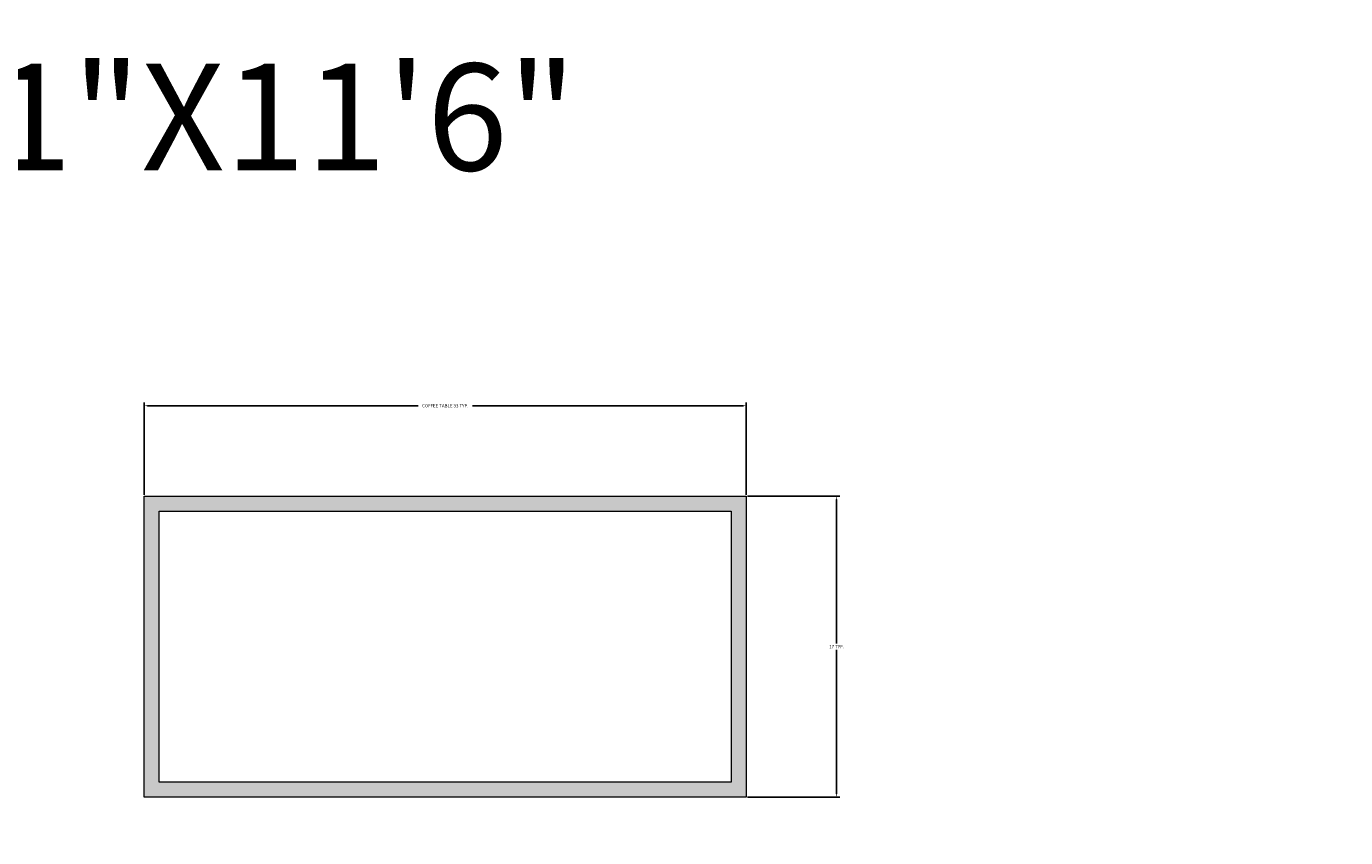
# Model space of a CAD drawing. Units: millimetres. Extents: x 27017497 to 27018854, y 7058029 to 7059154.
# Tile 36 of 91: x 27017677 to 27017750, y 7058341 to 7058386. Entities that reach past the tile are written whole.
import ezdxf

# ---------------------------------------------------------------- set-up
doc = ezdxf.new("R2010")
doc.units = ezdxf.units.MM
doc.layers.add('A-ANNO-DIMS', color=2, linetype='Continuous', lineweight=18)
doc.layers.add('A-FURN', color=8, linetype='Continuous', lineweight=18)
doc.layers.add('A-FURN-PATT', color=177, linetype='Continuous', lineweight=13, true_color=0x293189)
doc.styles.get("Standard").update_dxf_attribs({"font": 'arial.ttf'})
doc.dimstyles.get("Standard").update_dxf_attribs({"dimtxt": 0.18, "dimasz": 0.18, "dimexe": 0.18, "dimexo": 0.0625, "dimgap": 0.09, "dimtad": 0, "dimtih": 1, "dimtoh": 1, "dimdec": 4, "dimzin": 0, "dimdsep": 46, "dimtxsty": 'Standard', "dimcen": 0.09, "dimadec": 0, "dimazin": 0, "dimtfac": 1, "dimtdec": 4, "dimtofl": 0, "dimtmove": 0, "dimatfit": 3, "dimfxl": 1, "dimtolj": 1, "dimtzin": 0, "dimarcsym": 0})

# ---------------------------------------------------------------- blocks, each defined once
blk = doc.blocks.new('TABLE-COFFEE')
for p, q in [((33.345, 16.673), (0, 16.673)), ((0, 16.673), (0, 0)), ((33.345, 0), (33.345, 16.673)), ((32.511, 15.839), (0.834, 15.839)), ((0.834, 15.839), (0.834, 0.834)), ((32.511, 0.834), (32.511, 15.839)), ((0.834, 0.834), (32.511, 0.834)), ((0, 0), (33.345, 0))]:
    blk.add_line(p, q)
blk = doc.blocks.new('*D31')
at = {"layer": 'A-ANNO-DIMS', "color": 0, "lineweight": -2, "transparency": 16777216}
for p, q in [((27017683.615, 7058359.83), (27017683.615, 7058364.949)), ((27017683.795, 7058364.769), (27017698.783, 7058364.769)), ((27017716.78, 7058364.769), (27017701.793, 7058364.769)), ((27017716.96, 7058359.83), (27017716.96, 7058364.949))]:
    blk.add_line(p, q, dxfattribs=at)
at = {"layer": 'A-ANNO-DIMS', "color": 0, "transparency": 16777216}
for points in [[(27017683.795, 7058364.799), (27017683.795, 7058364.739), (27017683.615, 7058364.769)], [(27017716.78, 7058364.799), (27017716.78, 7058364.739), (27017716.96, 7058364.769)]]:
    blk.add_solid(points, dxfattribs=at)
at = {"layer": 'Defpoints', "color": 0, "transparency": 16777216}
for p in [(27017716.96, 7058364.769), (27017683.615, 7058359.767), (27017716.96, 7058359.767)]:
    blk.add_point(p, dxfattribs=at)
at = {"layer": 'A-ANNO-DIMS', "color": 0, "transparency": 16777216, "insert": (27017700.288, 7058364.769), "char_height": 0.18, "attachment_point": 5}
blk.add_mtext('\\A1;COFFEE TABLE 33 TYP.', dxfattribs=at)
blk = doc.blocks.new('*D32')
at = {"layer": 'A-ANNO-DIMS', "color": 0, "lineweight": -2, "transparency": 16777216}
for p, q in [((27017717.023, 7058359.767), (27017722.142, 7058359.767)), ((27017721.962, 7058359.587), (27017721.962, 7058351.611)), ((27017721.962, 7058343.275), (27017721.962, 7058351.25)), ((27017717.023, 7058343.095), (27017722.142, 7058343.095))]:
    blk.add_line(p, q, dxfattribs=at)
at = {"layer": 'A-ANNO-DIMS', "color": 0, "transparency": 16777216}
for points in [[(27017721.932, 7058359.587), (27017721.992, 7058359.587), (27017721.962, 7058359.767)], [(27017721.932, 7058343.275), (27017721.992, 7058343.275), (27017721.962, 7058343.095)]]:
    blk.add_solid(points, dxfattribs=at)
at = {"layer": 'Defpoints', "color": 0, "transparency": 16777216}
for p in [(27017716.96, 7058359.767), (27017716.96, 7058343.095), (27017721.962, 7058343.095)]:
    blk.add_point(p, dxfattribs=at)
at = {"layer": 'A-ANNO-DIMS', "color": 0, "transparency": 16777216, "insert": (27017721.962, 7058351.431), "char_height": 0.18, "attachment_point": 5}
blk.add_mtext('\\A1;17 TYP.', dxfattribs=at)
blk = doc.blocks.new('*D48')
at = {"layer": 'A-ANNO-DIMS', "color": 0, "lineweight": -2, "transparency": 16777216}
for p, q in [((27018463.498, 7058622.912), (27017497.536, 7058622.912)), ((27017497.716, 7058622.732), (27017497.716, 7058357.753)), ((27017497.716, 7058092.41), (27017497.716, 7058357.389)), ((27018555.129, 7058092.23), (27017497.536, 7058092.23))]:
    blk.add_line(p, q, dxfattribs=at)
at = {"layer": 'A-ANNO-DIMS', "color": 0, "transparency": 16777216}
for points in [[(27017497.686, 7058622.732), (27017497.746, 7058622.732), (27017497.716, 7058622.912)], [(27017497.686, 7058092.41), (27017497.746, 7058092.41), (27017497.716, 7058092.23)]]:
    blk.add_solid(points, dxfattribs=at)
at = {"layer": 'Defpoints', "color": 0, "transparency": 16777216}
for p in [(27018463.561, 7058622.912), (27017497.716, 7058092.23), (27018555.192, 7058092.23)]:
    blk.add_point(p, dxfattribs=at)
at = {"layer": 'A-ANNO-DIMS', "color": 0, "transparency": 16777216, "insert": (27017497.716, 7058357.571), "char_height": 0.18, "attachment_point": 5}
blk.add_mtext('\\A1;530.7', dxfattribs=at)

msp = doc.modelspace()

# ---------------------------------------------------------------- hatches: boundary and pattern name
at = {"layer": 'A-FURN-PATT'}
h = msp.add_hatch(color=256, dxfattribs=at)
h.dxf.hatch_style = 1
h.paths.add_polyline_path([(27017716.96, 7058359.767), (27017683.615, 7058359.767), (27017683.615, 7058343.095), (27017716.96, 7058343.095)])
h.paths.add_polyline_path([(27017716.127, 7058358.933), (27017716.127, 7058343.928), (27017684.449, 7058343.928), (27017684.449, 7058358.933)], flags=16)
h.paths.add_polyline_path([(27017660.259, 7058359.819, 0.414214), (27017658.98, 7058361.098), (27017648.54, 7058361.098, 0.414214), (27017645.981, 7058358.539), (27017645.981, 7058344.31, 0.414214), (27017648.54, 7058341.751), (27017658.98, 7058341.751, 0.414214), (27017660.259, 7058343.031), (27017660.259, 7058344.31, 0.414214), (27017658.98, 7058345.59), (27017649.82, 7058345.59), (27017649.82, 7058353.053), (27017649.82, 7058357.26), (27017658.98, 7058357.26, 0.414214), (27017660.259, 7058358.539)])
h.paths.add_polyline_path([(27017664.147, 7058358.539, 0.414214), (27017661.588, 7058361.098), (27017658.98, 7058361.098, -0.414214), (27017660.259, 7058359.819), (27017660.259, 7058358.539, -0.414214), (27017658.98, 7058357.26), (27017650.587, 7058357.26, -0.414214), (27017651.099, 7058356.748), (27017651.099, 7058356.283), (27017651.099, 7058346.869, 0.414214), (27017652.379, 7058345.59), (27017658.98, 7058345.59, -0.414214), (27017660.259, 7058344.31), (27017660.259, 7058343.031, -0.414214), (27017658.98, 7058341.751), (27017661.588, 7058341.751, 0.414214), (27017664.147, 7058344.31)])
h.paths.add_polyline_path([(27017651.099, 7058356.283), (27017651.099, 7058356.748, 0.414214), (27017650.587, 7058357.26), (27017650.331, 7058357.26, 0.414214), (27017649.82, 7058356.748), (27017649.82, 7058346.101, 0.414214), (27017650.331, 7058345.59), (27017650.587, 7058345.59, 0.414214), (27017651.099, 7058346.101)], flags=17)

# ---------------------------------------------------------------- block references
at = {"layer": 'A-FURN', "extrusion": (0, 0, -1), "zscale": -1, "rotation": 180}
msp.add_blockref('TABLE-COFFEE', (-27017683.615, 7058359.767), dxfattribs=at)

# ---------------------------------------------------------------- texts
at = {"layer": 'A-ANNO-DIMS'}
msp.add_text('10\'1"X11\'6"', height=5.91176, dxfattribs=at).set_placement((27017663.959, 7058377.8))

# ---------------------------------------------------------------- dimensions: what is measured, and where the dimension line sits
dim = msp.add_linear_dim(base=(27017497.716, 7058092.23), p1=(27018463.561, 7058622.912), p2=(27018555.192, 7058092.23), angle=90, dimstyle='Standard', override={"dimdec": 1, "dimlfac": 1, "dimrnd": 0, "dimzin": 0, "dimdsep": 46, "dimlunit": 2}, dxfattribs=at)
dim.commit()
dim.dimension.update_dxf_attribs({"geometry": '*D48', "text_midpoint": (27017497.716, 7058357.571)})
dim = msp.add_linear_dim(base=(27017716.96, 7058364.769), p1=(27017683.615, 7058359.767), p2=(27017716.96, 7058359.767), text='COFFEE TABLE <> TYP.', dimstyle='Standard', override={"dimdec": 0, "dimlfac": 1, "dimrnd": 0, "dimzin": 0, "dimdsep": 46, "dimlunit": 2}, dxfattribs=at)
dim.commit()
dim.dimension.update_dxf_attribs({"geometry": '*D31', "text_midpoint": (27017700.288, 7058364.769)})
dim = msp.add_linear_dim(base=(27017721.962, 7058343.095), p1=(27017716.96, 7058359.767), p2=(27017716.96, 7058343.095), angle=270, text='<> TYP.', dimstyle='Standard', override={"dimdec": 0, "dimlfac": 1, "dimrnd": 0, "dimzin": 0, "dimdsep": 46, "dimlunit": 2}, dxfattribs=at)
dim.commit()
dim.dimension.update_dxf_attribs({"geometry": '*D32', "text_midpoint": (27017721.962, 7058351.431)})

doc.saveas('drawing.dxf')
